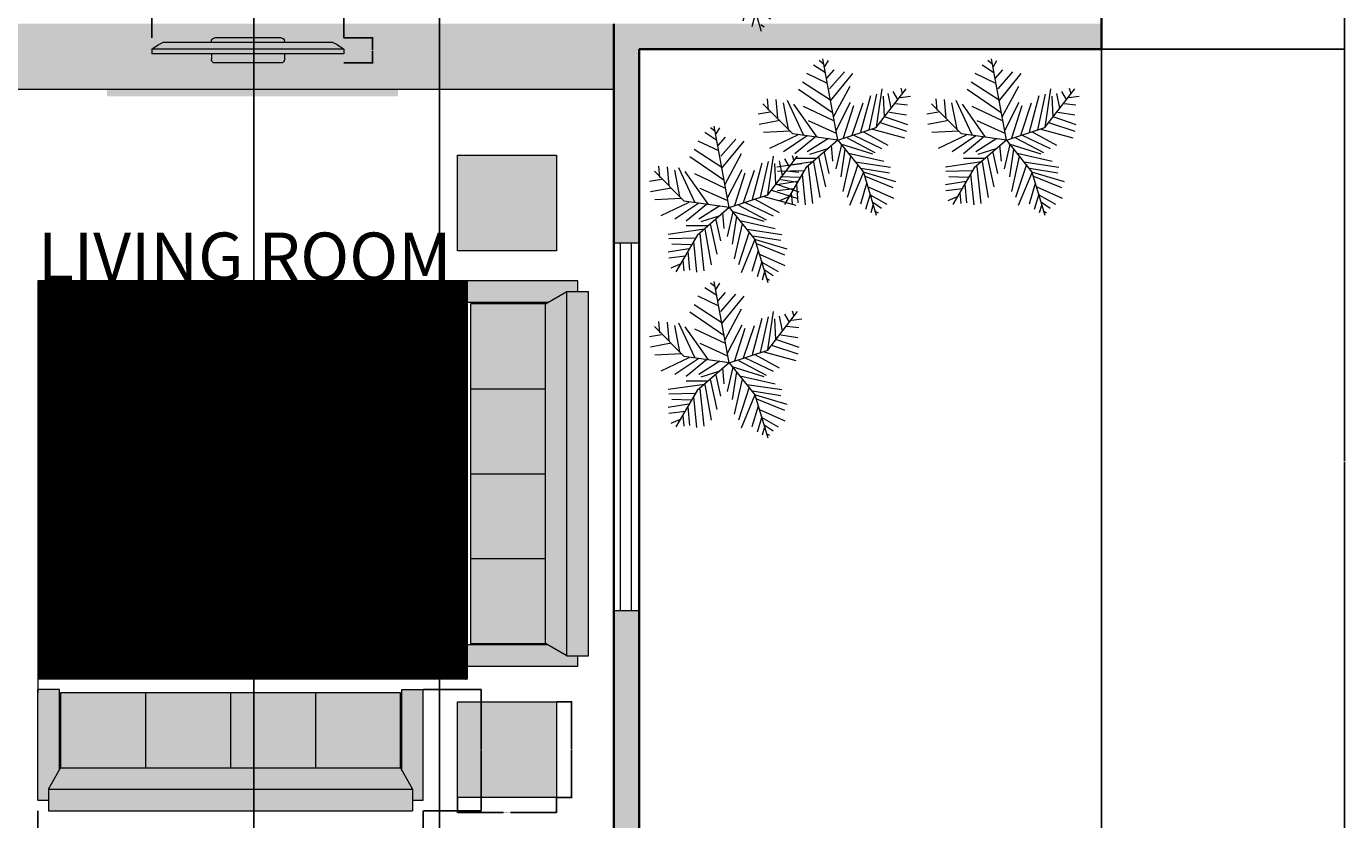
# Model space of a CAD drawing. Units: inches. Extents: x 192 to 1361, y -1362 to 367.
# Tile 12 of 23: x 891 to 1361, y -1057 to -775. Entities that reach past the tile are written whole.
import ezdxf

# ---------------------------------------------------------------- set-up
doc = ezdxf.new("R2010")
doc.units = ezdxf.units.IN
doc.header["$MEASUREMENT"] = 0
for name, color, linetype, lineweight in [('A-ANNO-DIMS', 2, 'Continuous', 18), ('A-AREA-IDEN', 7, 'Continuous', 18), ('A-EQPM', 8, 'Continuous', 18), ('A-FLOR', 8, 'Continuous', 18), ('A-FLOR-CASE', 32, 'Continuous', 18), ('A-WALL-PATT', 250, 'Continuous', 13), ('furniture', 32, 'Continuous', 18), ('lawn', 96, 'Continuous', 13), ('walls', 7, 'Continuous', 35), ('windows', 4, 'Continuous', 18)]:
    doc.layers.add(name, color=color, linetype=linetype, lineweight=lineweight)
for name, color, linetype, lineweight, true_color in [('A-EQPM-PATT', 251, 'Continuous', 13, 0x636466), ('A-FLOR-CASE-PATT', 9, 'Continuous', 13, 0xc7c8ca), ('A-FLOR-PATT', 254, 'Continuous', 13, 0xfeeab9), ('A-FURN-PATT', 254, 'Continuous', 13, 0xfeeab9)]:
    doc.layers.add(name, color=color, linetype=linetype, lineweight=lineweight, true_color=true_color)
doc.styles.get("Standard").update_dxf_attribs({"font": 'arial.ttf'})
doc.dimstyles.get("Standard").update_dxf_attribs({"dimtxt": 0.18, "dimasz": 0.18, "dimexe": 0.18, "dimexo": 0.0625, "dimgap": 0.09, "dimtad": 0, "dimtih": 1, "dimtoh": 1, "dimzin": 0, "dimdsep": 46, "dimlunit": 3, "dimtxsty": 'Standard', "dimcen": 0.09, "dimadec": 0, "dimazin": 0, "dimtfac": 1, "dimtofl": 0, "dimtmove": 0, "dimatfit": 3, "dimfxl": 1, "dimtolj": 1, "dimtzin": 0, "dimarcsym": 0})

# ---------------------------------------------------------------- blocks, each defined once
blk = doc.blocks.new('*U4')
for p, q in [((-10.186, 53.64), (-13.084, 55.962)), ((0, 0), (-10.5, 57)), ((-9.099, 51.782), (-6.563, 55.962)), ((-8.737, 47.138), (-17.069, 52.711)), ((-7.65, 43.423), (-2.578, 49.46)), ((-5.839, 35.992), (4.667, 48.067)), ((-7.288, 39.707), (-21.778, 46.673)), ((-5.114, 27.632), (10.463, 46.673)), ((-5.114, 28.097), (-24.676, 40.636)), ((-2.941, 16.486), (8.652, 37.85)), ((-3.665, 19.273), (-27.574, 35.527)), ((22.055, 7.198), (27.489, 32.277)), ((27, 9), (48, 36)), ((27.127, 9.056), (31.112, 35.992)), ((35.096, 32.741), (37.27, 22.524)), ((38.719, 34.134), (41.979, 28.561)), ((44.153, 36.456), (45.239, 32.741)), ((-48.585, 21.131), (-49.309, 29.026)), ((-43.513, 28.561), (-42.427, 15.558)), ((-35.544, 28.097), (-24.314, 3.947)), ((-1.129, 6.734), (9.014, 26.704)), ((16.259, 5.805), (23.142, 31.348)), ((31.836, 30.883), (32.561, 16.486)), ((43.791, 29.954), (51.036, 30.883)), ((-31.5, 4.5), (-52.5, 25.5)), ((-38.442, 26.239), (-34.819, 7.663)), ((-14.533, 2.09), (-30.834, 25.31)), ((-24.314, 23.917), (-2.941, 13.7)), ((3.942, 1.625), (11.187, 24.381)), ((10.101, 3.483), (17.708, 26.239)), ((40.53, 25.775), (48.862, 24.846)), ((-47.498, 19.737), (-55.83, 18.344)), ((33.285, 16.486), (48.862, 10.913)), ((36.183, 19.737), (48.137, 17.88)), ((-40.615, 13.7), (-55.105, 10.913)), ((-20.691, 13.7), (-1.129, 4.876)), ((29.662, 12.307), (48.137, 6.269)), ((-33.37, 6.269), (-52.207, 5.34)), ((0, 0), (27, 9)), ((18.07, 5.805), (35.096, -3.483)), ((24.229, 7.663), (46.688, 1.625)), ((-28.299, 3.483), (-47.86, -5.805)), ((-21.416, 3.018), (-38.079, -8.128)), ((0, 0), (-31.5, 4.5)), ((-15.982, 2.09), (-30.11, -9.521)), ((0, 0), (-22.5, -19.5)), ((-6.563, 1.161), (-21.416, -8.128)), ((0, 0), (18, -22.5)), ((6.478, 1.625), (26.04, -8.592)), ((11.187, 3.483), (30.749, -5.805)), ((-4.752, -3.483), (-3.665, -14.629)), ((2.493, -3.019), (-1.491, -20.202)), ((1.769, -2.555), (24.229, -9.521)), ((-6.563, -5.805), (-19.967, -9.985)), ((-9.461, -8.592), (-6.201, -23.453)), ((5.029, -6.27), (2.131, -25.775)), ((7.565, -9.056), (32.198, -14.629)), ((-17.431, -15.094), (-42.789, -18.809)), ((-15.257, -12.772), (-30.11, -12.772)), ((-17.069, -15.094), (-12.721, -40.172)), ((-13.446, -11.378), (-8.737, -32.741)), ((9.014, -11.378), (3.58, -35.992)), ((12.274, -15.094), (36.907, -18.809)), ((-22.5, -19.5), (-37.5, -45)), ((-20.691, -18.345), (-17.793, -44.352)), ((14.085, -16.951), (6.478, -40.172)), ((16.259, -19.738), (36.183, -22.989)), ((-24.314, -21.596), (-42.427, -22.06)), ((-26.849, -26.24), (-40.253, -25.775)), ((-25.038, -23.918), (-22.865, -45.281)), ((18.07, -22.524), (8.289, -45.745)), ((18, -22.5), (27, -52.5)), ((18.433, -22.524), (40.53, -29.026)), ((19.157, -25.311), (38.719, -33.206)), ((-28.299, -29.026), (-42.789, -31.348)), ((-29.023, -30.884), (-27.936, -43.887)), ((20.244, -30.419), (15.897, -44.816)), ((-30.834, -34.135), (-42.427, -35.528)), ((-32.646, -36.921), (-31.921, -44.352)), ((21.331, -32.741), (39.081, -40.636)), ((-34.457, -39.708), (-40.978, -42.494)), ((22.78, -37.85), (19.519, -48.532)), ((22.78, -38.314), (34.372, -44.816)), ((24.591, -45.745), (23.142, -50.854)), ((24.591, -43.423), (30.749, -47.603)), ((26.764, -49.925), (28.213, -50.854))]:
    blk.add_line(p, q)
blk = doc.blocks.new('PLASMA-LARGE')
at = {"layer": 'furniture'}
for p, q in [((-7.26, 0), (7.26, 0)), ((-21, -2.5), (21, -2.5)), ((-21, -2.5), (-21, -3.5)), ((-18.61, -1), (18.61, -1)), ((-8, -1), (-8, -0.74)), ((8, -1), (8, -0.74)), ((21, -2.5), (21, -3.5)), ((-21, -3.5), (21, -3.5)), ((-8, -3.5), (-8, -4.76)), ((-7.26, -5.5), (7.26, -5.5)), ((8, -3.5), (8, -4.76))]:
    blk.add_line(p, q, dxfattribs=at)
for centre, radius, start, end in [((-7.26, -0.74), 0.744, 90, 180), ((7.26, -0.74), 0.744, 0, 90), ((-13.97, -11.05), 11.07, 114.7602, 129.4175), ((13.97, -11.05), 11.07, 50.5825, 65.2398), ((-7.26, -4.76), 0.744, 180, 270), ((7.26, -4.76), 0.744, 270, 0)]:
    blk.add_arc(centre, radius, start, end, dxfattribs=at)
blk = doc.blocks.new('FABRIC SOFA 4S')
at = {"layer": 'furniture'}
for p, q in [((3, 54), (34, 54)), ((3, 51), (3, 54)), ((34, 48), (34, 54)), ((0, -51), (0, 51)), ((6, 51), (0, 51)), ((6, -51), (6, 51)), ((12, 47.63), (6, 51)), ((11.14, 48), (34, 48)), ((33, 23.81), (12, 23.81)), ((33, 0), (12, 0)), ((33, -23.81), (12, -23.81)), ((6, -51), (12, -47.63)), ((11.54, -48), (34, -48)), ((34, -48), (34, -54)), ((6, -51), (0, -51)), ((3, -54), (3, -51)), ((3, -54), (34, -54))]:
    blk.add_line(p, q, dxfattribs=at)
blk.add_lwpolyline([(12, -47.63), (12, 47.63), (33, 47.63), (33, -47.63)], close=True, dxfattribs=at)
blk = doc.blocks.new('LIVING-SIDE-TABLE')
for p, q in [((0, 34.07), (35.35, 34.07)), ((0, 0), (0, 34.07)), ((35.35, 34.07), (35.35, 0)), ((35.35, 0), (0, 0))]:
    blk.add_line(p, q)
blk = doc.blocks.new('*D27')
at = {"layer": 'A-ANNO-DIMS', "color": 0, "lineweight": -2, "transparency": 16777216}
for p, q in [((894.63, -1054.34), (894.63, -1075.05)), ((1031.96, -1054.34), (1031.96, -1075.05)), ((894.81, -1074.87), (962.32, -1074.87)), ((1031.78, -1074.87), (964.27, -1074.87))]:
    blk.add_line(p, q, dxfattribs=at)
at = {"layer": 'A-ANNO-DIMS', "color": 0, "transparency": 16777216}
for points in [[(894.81, -1074.84), (894.81, -1074.9), (894.63, -1074.87)], [(1031.78, -1074.84), (1031.78, -1074.9), (1031.96, -1074.87)]]:
    blk.add_solid(points, dxfattribs=at)
at = {"layer": 'Defpoints', "color": 0, "transparency": 16777216}
for p in [(894.63, -1054.27), (1031.96, -1054.27), (1031.96, -1074.87)]:
    blk.add_point(p, dxfattribs=at)
at = {"layer": 'A-ANNO-DIMS', "color": 0, "transparency": 16777216, "insert": (963.29, -1074.87), "char_height": 0.18, "attachment_point": 5}
blk.add_mtext('\\A1;SOFA 137 TYP.', dxfattribs=at)
blk = doc.blocks.new('*D28')
at = {"layer": 'A-ANNO-DIMS', "color": 0, "lineweight": -2, "transparency": 16777216}
for p, q in [((1032.02, -1011.04), (1052.74, -1011.04)), ((1052.56, -1011.22), (1052.56, -1032.47)), ((1052.56, -1054.09), (1052.56, -1032.84)), ((1032.02, -1054.27), (1052.74, -1054.27))]:
    blk.add_line(p, q, dxfattribs=at)
at = {"layer": 'A-ANNO-DIMS', "color": 0, "transparency": 16777216}
for points in [[(1052.53, -1011.22), (1052.59, -1011.22), (1052.56, -1011.04)], [(1052.53, -1054.09), (1052.59, -1054.09), (1052.56, -1054.27)]]:
    blk.add_solid(points, dxfattribs=at)
at = {"layer": 'Defpoints', "color": 0, "transparency": 16777216}
for p in [(1031.96, -1011.04), (1052.56, -1011.04), (1031.96, -1054.27)]:
    blk.add_point(p, dxfattribs=at)
at = {"layer": 'A-ANNO-DIMS', "color": 0, "transparency": 16777216, "insert": (1052.56, -1032.66), "char_height": 0.18, "attachment_point": 5}
blk.add_mtext('\\A1;43 TYP.', dxfattribs=at)
blk = doc.blocks.new('*D39')
at = {"layer": 'A-ANNO-DIMS', "color": 0, "lineweight": -2, "transparency": 16777216}
for p, q in [((1044.12, -1049.62), (1044.12, -1055.04)), ((1079.46, -1049.62), (1079.46, -1055.04)), ((1044.3, -1054.86), (1060.5, -1054.86)), ((1079.28, -1054.86), (1063.08, -1054.86))]:
    blk.add_line(p, q, dxfattribs=at)
at = {"layer": 'A-ANNO-DIMS', "color": 0, "transparency": 16777216}
for points in [[(1044.3, -1054.83), (1044.3, -1054.89), (1044.12, -1054.86)], [(1079.28, -1054.83), (1079.28, -1054.89), (1079.46, -1054.86)]]:
    blk.add_solid(points, dxfattribs=at)
at = {"layer": 'Defpoints', "color": 0, "transparency": 16777216}
for p in [(1044.12, -1049.56), (1079.46, -1049.56), (1079.46, -1054.86)]:
    blk.add_point(p, dxfattribs=at)
at = {"layer": 'A-ANNO-DIMS', "color": 0, "transparency": 16777216, "insert": (1061.79, -1054.86), "char_height": 0.18, "attachment_point": 5}
blk.add_mtext('\\A1;SIDE TABLE 35 TYP.', dxfattribs=at)
blk = doc.blocks.new('*D40')
at = {"layer": 'A-ANNO-DIMS', "color": 0, "lineweight": -2, "transparency": 16777216}
for p, q in [((1079.53, -1015.5), (1084.95, -1015.5)), ((1084.77, -1015.68), (1084.77, -1032.35)), ((1084.77, -1049.38), (1084.77, -1032.71)), ((1079.53, -1049.56), (1084.95, -1049.56))]:
    blk.add_line(p, q, dxfattribs=at)
at = {"layer": 'A-ANNO-DIMS', "color": 0, "transparency": 16777216}
for points in [[(1084.74, -1015.68), (1084.8, -1015.68), (1084.77, -1015.5)], [(1084.74, -1049.38), (1084.8, -1049.38), (1084.77, -1049.56)]]:
    blk.add_solid(points, dxfattribs=at)
at = {"layer": 'Defpoints', "color": 0, "transparency": 16777216}
for p in [(1079.46, -1015.5), (1084.77, -1015.5), (1079.46, -1049.56)]:
    blk.add_point(p, dxfattribs=at)
at = {"layer": 'A-ANNO-DIMS', "color": 0, "transparency": 16777216, "insert": (1084.77, -1032.53), "char_height": 0.18, "attachment_point": 5}
blk.add_mtext('\\A1;34 TYP.', dxfattribs=at)
blk = doc.blocks.new('*D41')
at = {"layer": 'A-ANNO-DIMS', "color": 0, "lineweight": -2, "transparency": 16777216}
for p, q in [((935.27, -778.85), (935.27, -768.47)), ((935.45, -768.65), (969.03, -768.65)), ((1003.45, -768.65), (969.87, -768.65)), ((1003.63, -778.85), (1003.63, -768.47))]:
    blk.add_line(p, q, dxfattribs=at)
at = {"layer": 'A-ANNO-DIMS', "color": 0, "transparency": 16777216}
for points in [[(935.45, -768.62), (935.45, -768.68), (935.27, -768.65)], [(1003.45, -768.62), (1003.45, -768.68), (1003.63, -768.65)]]:
    blk.add_solid(points, dxfattribs=at)
at = {"layer": 'Defpoints', "color": 0, "transparency": 16777216}
for p in [(935.27, -768.65), (935.27, -778.91), (1003.63, -778.91)]:
    blk.add_point(p, dxfattribs=at)
at = {"layer": 'A-ANNO-DIMS', "color": 0, "transparency": 16777216, "insert": (969.45, -768.65), "char_height": 0.18, "attachment_point": 5}
blk.add_mtext('\\A1;TV 68', dxfattribs=at)
blk = doc.blocks.new('*D42')
at = {"layer": 'A-ANNO-DIMS', "color": 0, "lineweight": -2, "transparency": 16777216}
for p, q in [((1003.69, -778.91), (1014.07, -778.91)), ((1013.89, -779.09), (1013.89, -783.2)), ((1013.89, -787.68), (1013.89, -783.57)), ((1003.69, -787.86), (1014.07, -787.86))]:
    blk.add_line(p, q, dxfattribs=at)
at = {"layer": 'A-ANNO-DIMS', "color": 0, "transparency": 16777216}
for points in [[(1013.86, -779.09), (1013.92, -779.09), (1013.89, -778.91)], [(1013.86, -787.68), (1013.92, -787.68), (1013.89, -787.86)]]:
    blk.add_solid(points, dxfattribs=at)
at = {"layer": 'Defpoints', "color": 0, "transparency": 16777216}
for p in [(1003.63, -778.91), (1013.89, -778.91), (1003.63, -787.86)]:
    blk.add_point(p, dxfattribs=at)
at = {"layer": 'A-ANNO-DIMS', "color": 0, "transparency": 16777216, "insert": (1013.89, -783.38), "char_height": 0.18, "attachment_point": 5}
blk.add_mtext('\\A1;9', dxfattribs=at)
blk = doc.blocks.new('*D47')
at = {"layer": 'A-ANNO-DIMS', "color": 0, "lineweight": -2, "transparency": 16777216}
for p, q in [((1273.57, -782.95), (1273.57, -1200.05)), ((274.89, -914.5), (274.89, -1200.05)), ((275.07, -1199.87), (773.84, -1199.87)), ((1273.39, -1199.87), (774.62, -1199.87))]:
    blk.add_line(p, q, dxfattribs=at)
at = {"layer": 'A-ANNO-DIMS', "color": 0, "transparency": 16777216}
for points in [[(275.07, -1199.84), (275.07, -1199.9), (274.89, -1199.87)], [(1273.39, -1199.84), (1273.39, -1199.9), (1273.57, -1199.87)]]:
    blk.add_solid(points, dxfattribs=at)
at = {"layer": 'Defpoints', "color": 0, "transparency": 16777216}
for p in [(1273.57, -782.89), (274.89, -914.44), (1273.57, -1199.87)]:
    blk.add_point(p, dxfattribs=at)
at = {"layer": 'A-ANNO-DIMS', "color": 0, "transparency": 16777216, "insert": (774.23, -1199.87), "char_height": 0.18, "attachment_point": 5}
blk.add_mtext('\\A1;998.7', dxfattribs=at)
blk = doc.blocks.new('*D58')
at = {"layer": 'A-ANNO-DIMS', "color": 0, "lineweight": -2, "transparency": 16777216}
for p, q in [((1273.63, -597.5), (1360.41, -597.5)), ((1360.23, -597.68), (1360.23, -690.01)), ((1360.23, -782.71), (1360.23, -690.38)), ((1273.63, -782.89), (1360.41, -782.89))]:
    blk.add_line(p, q, dxfattribs=at)
at = {"layer": 'A-ANNO-DIMS', "color": 0, "transparency": 16777216}
for points in [[(1360.2, -597.68), (1360.26, -597.68), (1360.23, -597.5)], [(1360.2, -782.71), (1360.26, -782.71), (1360.23, -782.89)]]:
    blk.add_solid(points, dxfattribs=at)
at = {"layer": 'Defpoints', "color": 0, "transparency": 16777216}
for p in [(1273.57, -597.5), (1273.57, -782.89), (1360.23, -782.89)]:
    blk.add_point(p, dxfattribs=at)
at = {"layer": 'A-ANNO-DIMS', "color": 0, "transparency": 16777216, "insert": (1360.23, -690.2), "char_height": 0.18, "attachment_point": 5}
blk.add_mtext('\\A1;185.4', dxfattribs=at)
blk = doc.blocks.new('*D59')
at = {"layer": 'A-ANNO-DIMS', "color": 0, "lineweight": -2, "transparency": 16777216}
for p, q in [((1273.63, -782.89), (1360.41, -782.89)), ((1360.23, -783.07), (1360.23, -929.58)), ((1360.23, -1076.44), (1360.23, -929.94)), ((1108.9, -1076.62), (1360.41, -1076.62))]:
    blk.add_line(p, q, dxfattribs=at)
at = {"layer": 'A-ANNO-DIMS', "color": 0, "transparency": 16777216}
for points in [[(1360.2, -783.07), (1360.26, -783.07), (1360.23, -782.89)], [(1360.2, -1076.44), (1360.26, -1076.44), (1360.23, -1076.62)]]:
    blk.add_solid(points, dxfattribs=at)
at = {"layer": 'Defpoints', "color": 0, "transparency": 16777216}
for p in [(1273.57, -782.89), (1360.23, -782.89), (1108.84, -1076.62)]:
    blk.add_point(p, dxfattribs=at)
at = {"layer": 'A-ANNO-DIMS', "color": 0, "transparency": 16777216, "insert": (1360.23, -929.76), "char_height": 0.18, "attachment_point": 5}
blk.add_mtext('\\A1;293.73', dxfattribs=at)
blk = doc.blocks.new('*D68')
at = {"layer": 'A-ANNO-DIMS', "color": 0, "lineweight": -2, "transparency": 16777216}
for p, q in [((856.57, -597.56), (856.57, -1200.05)), ((971.58, -597.56), (971.58, -1200.05)), ((856.75, -1199.87), (913.79, -1199.87)), ((971.4, -1199.87), (914.36, -1199.87))]:
    blk.add_line(p, q, dxfattribs=at)
at = {"layer": 'A-ANNO-DIMS', "color": 0, "transparency": 16777216}
for points in [[(856.75, -1199.84), (856.75, -1199.9), (856.57, -1199.87)], [(971.4, -1199.84), (971.4, -1199.9), (971.58, -1199.87)]]:
    blk.add_solid(points, dxfattribs=at)
at = {"layer": 'Defpoints', "color": 0, "transparency": 16777216}
for p in [(856.57, -597.5), (971.58, -597.5), (971.58, -1199.87)]:
    blk.add_point(p, dxfattribs=at)
at = {"layer": 'A-ANNO-DIMS', "color": 0, "transparency": 16777216, "insert": (914.07, -1199.87), "char_height": 0.18, "attachment_point": 5}
blk.add_mtext('\\A1;115', dxfattribs=at)
blk = doc.blocks.new('*D72')
at = {"layer": 'A-ANNO-DIMS', "color": 0, "lineweight": -2, "transparency": 16777216}
for p, q in [((835.08, -1067.56), (835.08, 367.39)), ((835.26, 367.21), (935.95, 367.21)), ((1037.58, 367.21), (936.88, 367.21)), ((1037.76, -1067.56), (1037.76, 367.39))]:
    blk.add_line(p, q, dxfattribs=at)
at = {"layer": 'A-ANNO-DIMS', "color": 0, "transparency": 16777216}
for points in [[(835.26, 367.24), (835.26, 367.18), (835.08, 367.21)], [(1037.58, 367.24), (1037.58, 367.18), (1037.76, 367.21)]]:
    blk.add_solid(points, dxfattribs=at)
at = {"layer": 'Defpoints', "color": 0, "transparency": 16777216}
for p in [(1037.76, 367.21), (835.08, -1067.62), (1037.76, -1067.62)]:
    blk.add_point(p, dxfattribs=at)
at = {"layer": 'A-ANNO-DIMS', "color": 0, "transparency": 16777216, "insert": (936.42, 367.21), "char_height": 0.18, "attachment_point": 5}
blk.add_mtext('\\A1;202.68', dxfattribs=at)

msp = doc.modelspace()

# ---------------------------------------------------------------- hatches: boundary and pattern name
at = {"layer": 'A-EQPM-PATT'}
h = msp.add_hatch(color=256, dxfattribs=at)
h.dxf.hatch_style = 1
h.paths.add_polyline_path([(919.2603, -799.7463), (919.2603, -775.7691), (1022.9846, -775.7691), (1022.9846, -799.7463)])
h.paths.add_polyline_path([(1003.6315, -784.6051), (1003.6315, -782.9774, 0.06404186), (999.7376, -780.5358), (982.4711, -780.5358), (982.4711, -780.1196, 0.41421356), (981.2595, -778.9081), (957.6389, -778.9081, 0.41421356), (956.4274, -780.1196), (956.4274, -780.5358), (939.1608, -780.5358, 0.06404186), (935.2669, -782.9774), (935.2669, -784.6051), (956.4274, -784.6051), (956.4274, -786.649, 0.41421356), (957.6389, -787.8606), (981.2595, -787.8606, 0.41421356), (982.4711, -786.649), (982.4711, -784.6051)], flags=16)
at = {"layer": 'A-FLOR-CASE-PATT'}
h = msp.add_hatch(color=256, dxfattribs=at)
h.dxf.hatch_style = 1
h.paths.add_polyline_path([(1099.8366, -773.892), (784.8041, -773.892), (784.8041, -797.1415), (1099.8366, -797.1415)])
at = {"layer": 'A-FLOR-PATT'}
h = msp.add_hatch(dxfattribs=at)
h.set_pattern_fill('ANSI31', color=256)
h.paths.add_polyline_path([(1047.5376, -865.5205), (894.6259, -865.5205), (894.6259, -1007.4555), (1047.5376, -1007.4555)])
at = {"layer": 'A-FURN-PATT'}
h = msp.add_hatch(color=256, dxfattribs=at)
h.dxf.hatch_style = 1
h.paths.add_polyline_path([(1079.4647, -1015.4962), (1044.116, -1015.4962), (1044.116, -1049.5621), (1079.4647, -1049.5621)])
h.paths.add_polyline_path([(1079.4647, -820.7233), (1044.116, -820.7233), (1044.116, -854.7892), (1079.4647, -854.7892)])
h = msp.add_hatch(color=256, dxfattribs=at)
h.dxf.hatch_style = 1
h.paths.add_polyline_path([(1075.5123, -964.4652), (1048.8092, -964.4652), (1048.8092, -994.7446), (1075.5123, -994.7446)], flags=16)
h.paths.add_polyline_path([(1075.5123, -934.1857), (1048.8092, -934.1857), (1048.8092, -964.4652), (1075.5123, -964.4652)], flags=17)
h.paths.add_polyline_path([(1075.5123, -903.9062), (1048.8092, -903.9062), (1048.8092, -934.1857), (1075.5123, -934.1857)], flags=17)
h.paths.add_polyline_path([(1075.5123, -873.6268), (1048.8092, -873.6268), (1048.8092, -903.9062), (1075.5123, -903.9062)], flags=17)
h.paths.add_polyline_path([(1086.9565, -865.5205), (1047.5376, -865.5205), (1047.5376, -873.1499), (1076.36, -873.1499), (1083.1418, -869.3352), (1086.9565, -869.3352)], flags=17)
h.paths.add_polyline_path([(1083.1418, -869.3352), (1075.5123, -873.6268), (1075.5123, -994.7446), (1083.1418, -999.0362)], flags=16)
h.paths.add_polyline_path([(1090.7712, -869.3352), (1083.1418, -869.3352), (1083.1418, -999.0362), (1090.7712, -999.0362)], flags=17)
h.paths.add_polyline_path([(1075.5123, -994.7446), (1048.8092, -994.7446), (1048.8092, -964.4652), (1075.5123, -964.4652), (1075.5123, -873.6268), (1076.36, -873.1499), (1047.5376, -873.1499), (1047.5376, -865.5205), (1086.9565, -865.5205), (1086.9565, -869.3352), (1090.7712, -869.3352), (1090.7712, -999.0362), (1086.9565, -999.0362), (1086.9565, -1002.8509), (1047.5376, -1002.8509), (1047.5376, -995.2215), (1076.36, -995.2215)])
h = msp.add_hatch(color=256, dxfattribs=at)
h.dxf.hatch_style = 1
h.paths.add_polyline_path([(1075.5123, -964.4652), (1048.8092, -964.4652), (1048.8092, -994.7446), (1075.5123, -994.7446)])
h.paths.add_polyline_path([(1083.1418, -869.3352), (1075.5123, -873.6268), (1075.5123, -994.7446), (1083.1418, -999.0362)])
h.paths.add_polyline_path([(1090.7712, -869.3352), (1083.1418, -869.3352), (1083.1418, -999.0362), (1090.7712, -999.0362)])
h.paths.add_polyline_path([(1083.1418, -869.3352), (1086.9565, -869.3352), (1086.9565, -865.5205), (1047.5376, -865.5205), (1047.5376, -873.1499), (1076.36, -873.1499)])
h = msp.add_hatch(color=256, dxfattribs=at)
h.dxf.hatch_style = 1
h.paths.add_polyline_path([(942.4573, -943.9325), (942.4573, -921.9658), (956.3155, -921.9658), (956.3155, -917.6995), (942.4573, -917.6995), (942.4573, -913.7375), (996.317, -913.7375), (996.317, -933.9446), (981.7876, -933.9446), (981.7876, -938.211), (996.317, -938.211), (996.317, -943.9325)])
h.paths.add_polyline_path([(968.1537, -928.2906), (968.0828, -928.2408), (968.1371, -928.1746)], flags=16)
h.paths.add_polyline_path([(966.3531, -925.1502), (967.7671, -926.5641), (967.7728, -926.4479), (967.6213, -926.4184), (966.5175, -925.3145), (966.542, -925.1675)], flags=16)
h.paths.add_polyline_path([(971.8563, -931.717), (971.8661, -931.714), (971.8701, -931.7211)], flags=16)
h.paths.add_polyline_path([(965.7725, -929.1798), (965.7984, -929.1586), (968.3447, -929.6277), (968.0361, -930.5537), (967.9831, -930.5714), (968.0107, -930.6297), (967.5161, -932.1136), (966.8559, -932.6271), (966.8025, -932.6244), (966.8149, -932.659), (967.4987, -932.1271), (967.5122, -932.1251), (968.3447, -929.6277), (968.5904, -929.8243), (968.6021, -929.862), (968.6296, -929.8556), (969.7313, -930.737), (969.7665, -930.9701), (969.9482, -930.9105), (970.4039, -931.275), (970.4098, -931.2951), (970.4224, -931.2898), (968.3447, -929.6277), (969.7104, -928.052), (969.7297, -928.0553), (969.7342, -928.0244), (968.3447, -929.6277), (965.7537, -929.1504)], flags=16)
h.paths.add_polyline_path([(944.8189, -940.5185, 1), (944.8189, -942.0782, 1)], flags=16)
h = msp.add_hatch(color=256, dxfattribs=at)
h.dxf.hatch_style = 1
h.paths.add_polyline_path([(942.4573, -921.9658), (942.4573, -917.6995), (956.3155, -917.6995), (956.3155, -921.9658)])
h.paths.add_polyline_path([(938.6349, -921.9658), (938.6349, -917.6995), (942.4573, -917.6995), (942.4573, -921.9658)])
h.paths.add_polyline_path([(981.7876, -938.211), (981.7876, -933.9446), (996.317, -933.9446), (996.317, -938.211)])
h.paths.add_polyline_path([(996.317, -938.211), (996.317, -933.9446), (999.4682, -933.9446), (999.4682, -938.211)])
h = msp.add_hatch(color=256, dxfattribs=at)
h.dxf.hatch_style = 1
h.paths.add_polyline_path([(898.4406, -1046.6435), (1028.1416, -1046.6435), (1024.3268, -1039.8618), (1024.3268, -1011.0394), (1031.9563, -1011.0394), (1031.9563, -1050.4583), (1028.1416, -1050.4583), (1028.1416, -1054.273), (898.4406, -1054.273), (898.4406, -1050.4583), (894.6259, -1050.4583), (894.6259, -1011.0394), (902.2553, -1011.0394), (902.2553, -1039.8618)])
h = msp.add_hatch(color=256, dxfattribs=at)
h.dxf.hatch_style = 1
h.paths.add_polyline_path([(933.0116, -1012.3109), (902.7322, -1012.3109), (902.7322, -1039.0141), (933.0116, -1039.0141)])
h.paths.add_polyline_path([(963.2911, -1012.3109), (933.0116, -1012.3109), (933.0116, -1039.0141), (963.2911, -1039.0141)])
h.paths.add_polyline_path([(993.5705, -1012.3109), (963.2911, -1012.3109), (963.2911, -1039.0141), (993.5705, -1039.0141)])
h.paths.add_polyline_path([(1023.85, -1012.3109), (993.5705, -1012.3109), (993.5705, -1039.0141), (1023.85, -1039.0141)])
h.paths.add_polyline_path([(1023.85, -1039.0141), (902.7322, -1039.0141), (898.4406, -1046.6435), (1028.1416, -1046.6435)])
h.paths.add_polyline_path([(1028.1416, -1046.6435), (898.4406, -1046.6435), (898.4406, -1054.273), (1028.1416, -1054.273)])
at = {"layer": 'A-WALL-PATT'}
h = msp.add_hatch(color=256, dxfattribs=at)
h.dxf.hatch_style = 1
h.paths.add_polyline_path([(309.5452, 191.102), (300.5452, 191.102), (300.5452, -126.898), (309.5452, -126.898), (309.5452, -117.898)])
h.paths.add_polyline_path([(420.798, 191.102), (337.3229, 191.102), (337.3229, 182.102), (420.798, 182.102)])
h.paths.add_polyline_path([(518.5452, 182.102), (625.4022, 182.102), (625.4022, 191.102), (509.5452, 191.102), (509.5452, 114.3262), (518.5452, 114.3262)])
h.paths.add_polyline_path([(842.5452, 191.102), (763.4438, 191.102), (763.4438, 182.102), (833.5452, 182.102), (833.5452, 161.1615), (836.8088, 161.1615), (842.5452, 161.1615)])
h.paths.add_polyline_path([(842.5452, -16.5675), (833.5452, -16.5675), (833.5452, -60.4996), (784.8041, -60.4996), (784.8041, -354.6796), (793.8041, -354.6796), (793.8041, -69.4996), (1094.1252, -69.4996), (1094.1252, -60.4996), (842.5452, -60.4996)])
h.paths.add_polyline_path([(518.5452, 36.602), (509.5452, 36.602), (509.5452, -117.898), (420.2204, -117.898), (420.2204, -126.898), (518.5452, -126.898)])
h.paths.add_polyline_path([(474.8041, -377.0384), (465.8041, -377.0384), (465.8041, -381.5384), (465.8041, -450.898), (537.5717, -450.898), (537.5717, -441.898), (474.8041, -441.898)])
h.paths.add_polyline_path([(1162.8041, -380.6763), (1204.3001, -380.6763), (1204.3001, -375.6763), (1195.1471, -375.6763), (1153.8041, -375.6763), (1153.8041, -448.4996), (856.5691, -448.4996), (856.5691, -457.4996), (1162.8041, -457.4996)])
h.paths.add_polyline_path([(1162.8041, -525.128), (1153.8041, -525.128), (1153.8041, -597.4996), (1162.8041, -597.4996)], flags=17)
h.paths.add_polyline_path([(1162.8041, -60.4996), (1153.8041, -60.4996), (1153.8041, -69.4996), (1153.8041, -177.4733), (1205.8889, -177.4733), (1205.8889, -172.4733), (1162.8041, -172.4733)])
h.paths.add_polyline_path([(980.5799, -525.686), (971.5799, -525.686), (971.5799, -597.4996), (980.5799, -597.4996)], flags=17)
h.paths.add_polyline_path([(856.5691, -448.4996), (798.7542, -448.4996), (784.8041, -448.4996), (784.8041, -457.4996), (847.5691, -457.4996), (847.5691, -597.4996), (784.8041, -597.4996), (784.8041, -606.4996), (1273.5658, -606.4996), (1273.5658, -597.4996), (856.5691, -597.4996)])
h.paths.add_polyline_path([(1273.5658, -773.892), (1099.8366, -773.892), (1099.8366, -851.9362), (1108.8366, -851.9362), (1108.8366, -782.892), (1273.5658, -782.892)])
h.paths.add_polyline_path([(1108.8366, -982.9214), (1099.8366, -982.9214), (1099.8366, -1067.6246), (1037.7563, -1067.6246), (1037.7563, -1076.6246), (1108.8366, -1076.6246)])
h.paths.add_polyline_path([(835.078, -1067.6246), (758.8458, -1067.6246), (758.8458, -940.2324), (749.8458, -940.2324), (749.8458, -963.172), (749.8458, -970.4644), (749.8458, -1076.6246), (835.078, -1076.6246)])
h.paths.add_polyline_path([(450.307, -1066.9838), (441.307, -1066.9838), (441.307, -1076.6246), (450.307, -1076.6246)])
h.paths.add_polyline_path([(492.8925, -756.4415), (274.8925, -756.4415), (274.8925, -765.4415), (492.8925, -765.4415)])
h.paths.add_polyline_path([(283.8925, -835.2244), (274.8925, -835.2244), (274.8925, -914.4415), (492.8925, -914.4415), (492.8925, -839.9415), (483.8925, -839.9415), (483.8925, -905.4415), (283.8925, -905.4415)])
h.paths.add_polyline_path([(283.8925, -441.898), (283.8925, -375.4296), (281.6021, -375.4296), (281.6021, -399.4121), (274.8925, -399.4121), (274.8925, -441.898), (274.8925, -684.5089), (283.8925, -684.5089)])

# ---------------------------------------------------------------- linework, layer by layer
at = {"layer": 'A-FLOR'}
for p, q in [((1047.5376, -865.5205), (894.6259, -865.5205)), ((894.6259, -865.5205), (894.6259, -1012.3109)), ((1047.5376, -865.5205), (1047.5376, -1007.4555)), ((1047.5376, -1007.4555), (894.6259, -1007.4555))]:
    msp.add_line(p, q, dxfattribs=at)
at = {"layer": 'A-FLOR-CASE'}
msp.add_line((784.8041, -797.1415), (1099.8366, -797.1415), dxfattribs=at)
at = {"layer": 'walls'}
for p, q in [((1273.5658, -597.4996), (1273.5658, -782.892)), ((1099.8366, -773.892), (1099.8366, -1067.6246)), ((1273.5658, -782.892), (1108.8366, -782.892)), ((1108.8366, -782.892), (1108.8366, -1076.6246))]:
    msp.add_line(p, q, dxfattribs=at)
at = {"layer": 'windows'}
for p, q in [((1099.8366, -851.9362), (1108.8366, -851.9362)), ((1102.1913, -982.9214), (1102.1913, -851.9362)), ((1106.1402, -982.9214), (1106.1402, -851.9362)), ((1099.8366, -982.9214), (1108.8366, -982.9214))]:
    msp.add_line(p, q, dxfattribs=at)

# ---------------------------------------------------------------- block references
at = {"layer": 'A-EQPM', "xscale": -1.627729972730456, "yscale": 1.627729972730456, "zscale": 1.627729972730456}
msp.add_blockref('PLASMA-LARGE', (969.4492, -778.9081), dxfattribs=at)
at = {"layer": 'furniture', "rotation": 180}
msp.add_blockref('LIVING-SIDE-TABLE', (1079.4646, -820.7234), dxfattribs=at)
at = {"layer": 'furniture', "xscale": -1.271578197200921, "yscale": 1.271578197200921, "zscale": 1.271578197200921}
for p, rotation in [((1090.7712, -934.1857), 359.9999999998928), ((963.2911, -1054.273), 269.9999999998931)]:
    msp.add_blockref('FABRIC SOFA 4S', p, dxfattribs=dict(at, rotation=rotation))
at = {"layer": 'furniture'}
msp.add_blockref('LIVING-SIDE-TABLE', (1044.116, -1049.562), dxfattribs=at)
at = {"layer": 'lawn'}
for p, xscale, yscale, zscale in [((1128.537, -730.122), 0.8828807890770264, 0.8828807890770264, 0.8828807890770264), ((1179.6567, -815.3754), 0.5078671948952364, 0.5078671948952364, 0.5078671948952364), ((1239.7119, -815.3754), 0.5078671948952364, 0.5078671948952364, 0.5078671948952364), ((1140.9544, -839.3727), 0.5078671948952364, 0.5078671948952364, 0.5078671948952364), ((1140.9544, -894.7), 0.5078671948952364, 0.5078671948952364, 0.5078671948952364)]:
    msp.add_blockref('*U4', p, dxfattribs=dict(at, xscale=xscale, yscale=yscale, zscale=zscale))
at = {"layer": 'lawn', "xscale": -0.0920718146463569, "yscale": 0.0920718146463569, "zscale": 0.0920718146463569, "rotation": 90}
msp.add_blockref('*U4', (968.3447, -929.6277), dxfattribs=at)

# ---------------------------------------------------------------- texts
at = {"layer": 'A-AREA-IDEN'}
for s, p in [('LIVING ROOM', (894.6259, -865.5205)), ('343X372', (931.2177, -894.35))]:
    msp.add_text(s, height=17.23824, dxfattribs=at).set_placement(p)

# ---------------------------------------------------------------- dimensions: what is measured, and where the dimension line sits
at = {"layer": 'A-ANNO-DIMS'}
for base, p1, p2, override, picture, middle in [((1037.7563, 367.2097), (835.078, -1067.6246), (1037.7563, -1067.6246), {"dimdec": 2, "dimlfac": 1, "dimrnd": 0, "dimzin": 0, "dimdsep": 46, "dimlunit": 2}, '*D72', (936.4171, 367.2097)), ((971.5799, -1199.8727), (856.5691, -597.4996), (971.5799, -597.4996), {"dimdec": 0, "dimlfac": 1, "dimrnd": 0, "dimzin": 0, "dimdsep": 46, "dimlunit": 2}, '*D68', (914.0745, -1199.8727)), ((1273.5658, -1199.8727), (274.8925, -914.4415), (1273.5658, -782.892), {"dimdec": 1, "dimlfac": 1, "dimrnd": 0, "dimzin": 0, "dimdsep": 46, "dimlunit": 2}, '*D47', (774.2292, -1199.8727))]:
    dim = msp.add_linear_dim(base=base, p1=p1, p2=p2, dimstyle='Standard', override=override, dxfattribs=at)
    dim.commit()
    dim.dimension.update_dxf_attribs({"geometry": picture, "text_midpoint": middle})
for base, p1, p2, override, picture, middle in [((1360.2331, -782.892), (1273.5658, -597.4996), (1273.5658, -782.892), {"dimdec": 1, "dimlfac": 1, "dimrnd": 0, "dimzin": 0, "dimdsep": 46, "dimlunit": 2}, '*D58', (1360.2331, -690.1958)), ((1013.8862, -778.9081), (1003.6315, -787.8606), (1003.6315, -778.9081), {"dimdec": 0, "dimlfac": 1, "dimrnd": 0, "dimzin": 0, "dimdsep": 46, "dimlunit": 2}, '*D42', (1013.8862, -783.3843)), ((1360.2331, -782.892), (1108.8366, -1076.6246), (1273.5658, -782.892), {"dimdec": 2, "dimlfac": 1, "dimrnd": 0, "dimzin": 0, "dimdsep": 46, "dimlunit": 2}, '*D59', (1360.2331, -929.7583))]:
    dim = msp.add_linear_dim(base=base, p1=p1, p2=p2, angle=90, dimstyle='Standard', override=override, dxfattribs=at)
    dim.commit()
    dim.dimension.update_dxf_attribs({"geometry": picture, "text_midpoint": middle})
for base, p1, p2, angle, text, picture, middle in [((935.2669, -768.6534), (1003.6315, -778.9081), (935.2669, -778.9081), 180, 'TV <>', '*D41', (969.4492, -768.6534)), ((1052.5559, -1011.0394), (1031.9563, -1054.273), (1031.9563, -1011.0394), 90, '<> TYP.', '*D28', (1052.5559, -1032.6562)), ((1084.767, -1015.4962), (1079.4647, -1049.5621), (1079.4647, -1015.4962), 90, '<> TYP.', '*D40', (1084.767, -1032.5292))]:
    dim = msp.add_linear_dim(base=base, p1=p1, p2=p2, angle=angle, text=text, dimstyle='Standard', override={"dimdec": 0, "dimlfac": 1, "dimrnd": 0, "dimzin": 0, "dimdsep": 46, "dimlunit": 2}, dxfattribs=at)
    dim.commit()
    dim.dimension.update_dxf_attribs({"geometry": picture, "text_midpoint": middle})
for base, p1, p2, text, picture, middle in [((1079.4647, -1054.8644), (1044.116, -1049.5621), (1079.4647, -1049.5621), 'SIDE TABLE <> TYP.', '*D39', (1061.7903, -1054.8644)), ((1031.9563, -1074.8726), (894.6259, -1054.273), (1031.9563, -1054.273), 'SOFA <> TYP.', '*D27', (963.2911, -1074.8726))]:
    dim = msp.add_linear_dim(base=base, p1=p1, p2=p2, text=text, dimstyle='Standard', override={"dimdec": 0, "dimlfac": 1, "dimrnd": 0, "dimzin": 0, "dimdsep": 46, "dimlunit": 2}, dxfattribs=at)
    dim.commit()
    dim.dimension.update_dxf_attribs({"geometry": picture, "text_midpoint": middle})

doc.saveas('drawing.dxf')
